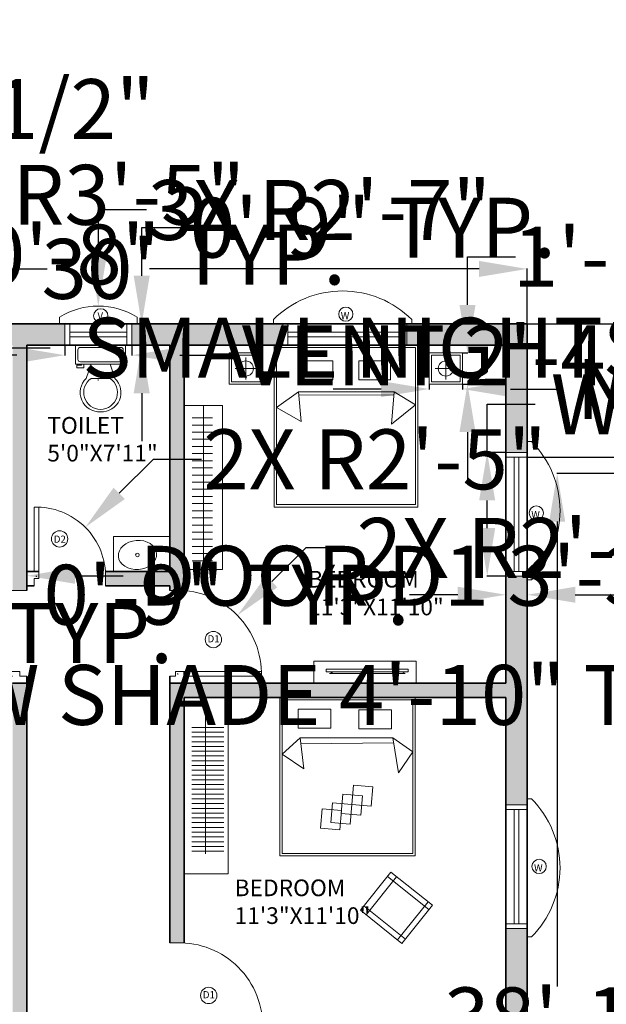
# Model space of a CAD drawing. Units: inches. Extents: x 28 to 3832, y 2 to 1709.
# Tile 4 of 7: x 2710 to 2956, y 1296 to 1709. Entities that reach past the tile are written whole.
import ezdxf

# ---------------------------------------------------------------- set-up
doc = ezdxf.new("R2010")
doc.units = ezdxf.units.IN
doc.header["$MEASUREMENT"] = 0
for name, color, linetype, lineweight in [('A-ANNO-DIMS', 2, 'Continuous', 18), ('A-ANNO-SYMB', 7, 'Continuous', 13), ('A-AREA-IDEN', 7, 'Continuous', 18), ('A-DOOR', 3, 'Continuous', 18), ('A-FLOR-CASE', 8, 'Continuous', 18), ('A-FLOR-CASE-PATT', 8, 'Continuous', 13), ('A-FLOR-FIXT', 9, 'Continuous', 18), ('A-FURN', 8, 'Continuous', 18), ('A-GLAZ', 4, 'Continuous', 18), ('A-ROOF-SHAD', 7, 'Continuous', 13), ('A-WALL', 7, 'Continuous', 35)]:
    doc.layers.add(name, color=color, linetype=linetype, lineweight=lineweight)
doc.layers.add('A-WALL-PATT', color=30, linetype='Continuous', lineweight=9, true_color=0xf26722)
doc.styles.get("Standard").update_dxf_attribs({"font": 'arial.ttf'})
doc.dimstyles.get("Standard").update_dxf_attribs({"dimtxt": 25.18, "dimasz": 20.18, "dimexe": 0.18, "dimexo": 0.0625, "dimgap": 0.09, "dimtad": 0, "dimtih": 1, "dimtoh": 1, "dimdec": 0, "dimzin": 0, "dimdsep": 46, "dimlunit": 3, "dimtxsty": 'Standard', "dimcen": 0.09, "dimadec": 0, "dimazin": 0, "dimtfac": 1, "dimtdec": 0, "dimtofl": 0, "dimtmove": 0, "dimatfit": 3, "dimfxl": 1, "dimtolj": 1, "dimtzin": 0, "dimarcsym": 0})

# ---------------------------------------------------------------- blocks, each defined once
blk = doc.blocks.new('*D1')
at = {"layer": 'A-ANNO-DIMS', "color": 0, "lineweight": -2, "transparency": 16777216}
for p, q in [((2562.64, 1581.59), (2562.64, 1604.74)), ((2582.82, 1604.56), (2721.19, 1604.56)), ((2902.46, 1604.56), (2764.09, 1604.56)), ((2922.64, 1581.59), (2922.64, 1604.74))]:
    blk.add_line(p, q, dxfattribs=at)
at = {"layer": 'A-ANNO-DIMS', "color": 0, "transparency": 16777216}
for points in [[(2582.82, 1607.92), (2582.82, 1601.2), (2562.64, 1604.56)], [(2902.46, 1607.92), (2902.46, 1601.2), (2922.64, 1604.56)]]:
    blk.add_solid(points, dxfattribs=at)
at = {"layer": 'Defpoints', "color": 0, "transparency": 16777216}
for p in [(2922.64, 1604.56), (2562.64, 1581.52), (2922.64, 1581.52)]:
    blk.add_point(p, dxfattribs=at)
at = {"layer": 'A-ANNO-DIMS', "color": 0, "transparency": 16777216, "insert": (2742.64, 1604.56), "char_height": 25.18, "attachment_point": 5}
blk.add_mtext("\\A1;30'", dxfattribs=at)
blk = doc.blocks.new('*U4')
for p, q in [((9.5, -6), (9.5, -2)), ((-8, -8.5), (-8, -8)), ((-7, -8), (-7, -9.5)), ((-4, -8), (-6, -14)), ((4, -8), (6, -14)), ((-10, -8.5), (-8, -8.5)), ((-10, -9.5), (-10, -8.5)), ((-7, -9.5), (-10, -9.5)), ((4, -14), (-4, -14))]:
    blk.add_line(p, q)
blk.add_lwpolyline([(10.5, -8), (10.5, 0), (-10.5, 0), (-10.5, -8)], close=True)
for points in [[(-9.5, -2), (-9.5, -6)], [(8.5, -1), (-8.5, -1)], [(-8.5, -7), (8.5, -7)]]:
    blk.add_lwpolyline(points)
for centre, radius, start, end in [((-8.625, -1.875), 0.8839, 81.8699, 188.1301), ((8.625, -1.875), 0.8839, 351.8699, 98.1301), ((-8.625, -6.125), 0.8839, 171.869898, 278.1301), ((8.625, -6.125), 0.8839, 261.8699, 8.1301), ((-0.4772, -19.9188), 8.0953, 133.01722, 273.38), ((0.0374, -19.8731), 7.127, 124.50543, 269.7), ((-0.0373, -19.8731), 7.127, 270.3, 55.4946), ((0.4773, -19.9188), 8.0953, 266.62, 46.9828)]:
    blk.add_arc(centre, radius, start, end)
blk = doc.blocks.new('DOOR-D1-36')
for p, q in [((33.01, 36), (39.01, 36)), ((36.01, 2), (0.01, 2)), ((33.01, 0), (0.01, 0)), ((36.01, 2), (36.01, 0)), ((36.01, 0), (39.01, 0))]:
    blk.add_line(p, q)
blk.add_arc((35.01, 1), 35.01, 88.3634, 181.6366)
blk = doc.blocks.new('DOOR-D2-30')
for p, q in [((0, 6), (0, 33)), ((2, 3), (2, 33)), ((30, 6), (30, 0)), ((2, 3), (0, 3)), ((0, 3), (0, 0))]:
    blk.add_line(p, q)
blk.add_arc((1, 4), 29.02, 358.0251, 91.9749)
blk = doc.blocks.new('WINDOW-48')
for p, q in [((0, 0), (0, 9)), ((2, 0), (2, 9)), ((50, 0), (50, 9)), ((52, 0), (52, 9)), ((2, 5.5), (50, 5.5)), ((2, 3.5), (50, 3.5))]:
    blk.add_line(p, q)
blk = doc.blocks.new('VENT-24')
for p, q in [((0, 0), (0, 9)), ((2, 0), (2, 9)), ((26, 0), (26, 9)), ((28, 0), (28, 9)), ((2, 5.5), (26, 5.5)), ((2, 3.5), (26, 3.5))]:
    blk.add_line(p, q)
blk = doc.blocks.new('WINDOW-SHADE')
for p, q in [((0, 1.76), (0, 0)), ((58.03, 1.76), (58.03, 0))]:
    blk.add_line(p, q)
blk.add_arc((29.02, -27.22), 41.01, 44.9571, 135.0429)
blk = doc.blocks.new('VENT-SHADE')
for p, q in [((0, 2.83), (0, 0)), ((32.5, 2.83), (32.5, 0))]:
    blk.add_line(p, q)
blk.add_arc((16.25, -23.61), 31.04, 58.4311, 121.5689)
blk = doc.blocks.new('BEDSIDE-TABLE')
for p, q in [((6.98, 11.18), (6.98, 1.93)), ((2.5, 6.54), (11.72, 6.54))]:
    blk.add_line(p, q)
for points in [[(0, 13.08), (13.97, 13.08), (13.97, 0), (0, 0)], [(1, 12.08), (12.97, 12.08), (12.97, 1), (1, 1)]]:
    blk.add_lwpolyline(points, close=True)
blk.add_circle((6.98, 6.54), 3.18)
blk = doc.blocks.new('OPENING-TAG-W')
blk.add_circle((3, 3), 3)
at = {"insert": (0.88, 3.88), "char_height": 3, "attachment_point": 1}
blk.add_mtext_dynamic_manual_height_columns('W', width=16.2124, gutter_width=1, heights=[0], dxfattribs=at)
blk = doc.blocks.new('OPENING-TAG-V')
blk.add_circle((3, 3), 3)
at = {"insert": (1.61, 4.52), "char_height": 3, "attachment_point": 1}
blk.add_mtext_dynamic_manual_height_columns('V', width=16.2124, gutter_width=1, heights=[0], dxfattribs=at)
blk = doc.blocks.new('OPENING-TAG-D1')
blk.add_circle((3.43, 3.43), 3.43)
at = {"insert": (0.97, 5.25), "char_height": 3, "attachment_point": 1}
blk.add_mtext_dynamic_manual_height_columns('D1', width=16.2124, gutter_width=1, heights=[0], dxfattribs=at)
blk = doc.blocks.new('OPENING-TAG-D2')
blk.add_circle((3.43, 3.43), 3.43)
at = {"insert": (0.96, 4.81), "char_height": 3, "attachment_point": 1}
blk.add_mtext_dynamic_manual_height_columns('D2', width=16.2124, gutter_width=1, heights=[0], dxfattribs=at)
blk = doc.blocks.new('*D23')
at = {"layer": 'A-ANNO-DIMS', "color": 0, "lineweight": -2, "transparency": 16777216}
for p, q in [((2540.14, 1405.47), (2540.14, 1425.65)), ((2540.14, 1425.65), (2560.32, 1425.65)), ((2548.79, 1405.47), (2539.96, 1405.47)), ((2540.14, 1367.62), (2540.14, 1385.29)), ((2548.79, 1347.44), (2539.96, 1347.44))]:
    blk.add_line(p, q, dxfattribs=at)
at = {"layer": 'A-ANNO-DIMS', "color": 0, "transparency": 16777216}
for points in [[(2536.78, 1385.29), (2543.51, 1385.29), (2540.14, 1405.47)], [(2536.78, 1367.62), (2543.51, 1367.62), (2540.14, 1347.44)]]:
    blk.add_solid(points, dxfattribs=at)
at = {"layer": 'Defpoints', "color": 0, "transparency": 16777216}
for p in [(2540.14, 1405.47), (2548.85, 1405.47), (2548.85, 1347.44)]:
    blk.add_point(p, dxfattribs=at)
at = {"layer": 'A-ANNO-DIMS', "color": 0, "transparency": 16777216, "insert": (2795, 1425.65), "char_height": 25.18, "attachment_point": 5}
blk.add_mtext('\\A1;WINDOW SHADE 4\'-10" TYP.', dxfattribs=at)
blk = doc.blocks.new('*D25')
at = {"layer": 'A-ANNO-DIMS', "color": 0, "lineweight": -2, "transparency": 16777216}
for p, q in [((2905.84, 1527.52), (2905.84, 1547.7)), ((2905.84, 1547.7), (2926.02, 1547.7)), ((2913.58, 1527.52), (2905.66, 1527.52)), ((2905.84, 1495.7), (2905.84, 1507.34)), ((2913.58, 1475.52), (2905.66, 1475.52))]:
    blk.add_line(p, q, dxfattribs=at)
at = {"layer": 'A-ANNO-DIMS', "color": 0, "transparency": 16777216}
for points in [[(2902.48, 1507.34), (2909.2, 1507.34), (2905.84, 1527.52)], [(2902.48, 1495.7), (2909.2, 1495.7), (2905.84, 1475.52)]]:
    blk.add_solid(points, dxfattribs=at)
at = {"layer": 'Defpoints', "color": 0, "transparency": 16777216}
for p in [(2905.84, 1527.52), (2913.64, 1527.52), (2913.64, 1475.52)]:
    blk.add_point(p, dxfattribs=at)
at = {"layer": 'A-ANNO-DIMS', "color": 0, "transparency": 16777216, "insert": (3085.42, 1547.7), "char_height": 25.18, "attachment_point": 5}
blk.add_mtext('\\A1;WINDOW 4\'-4" TYP.', dxfattribs=at)
blk = doc.blocks.new('*D26')
at = {"layer": 'A-ANNO-DIMS', "color": 0, "lineweight": -2, "transparency": 16777216}
for p, q in [((2913.64, 1475.46), (2913.64, 1467.54)), ((2922.64, 1475.46), (2922.64, 1467.54)), ((2893.46, 1467.72), (2873.28, 1467.72)), ((2942.82, 1467.72), (2963, 1467.72))]:
    blk.add_line(p, q, dxfattribs=at)
at = {"layer": 'A-ANNO-DIMS', "color": 0, "transparency": 16777216}
for points in [[(2893.46, 1471.09), (2893.46, 1464.36), (2913.64, 1467.72)], [(2942.82, 1471.09), (2942.82, 1464.36), (2922.64, 1467.72)]]:
    blk.add_solid(points, dxfattribs=at)
at = {"layer": 'Defpoints', "color": 0, "transparency": 16777216}
for p in [(2913.64, 1475.52), (2922.64, 1475.52), (2913.64, 1467.72)]:
    blk.add_point(p, dxfattribs=at)
at = {"layer": 'A-ANNO-DIMS', "color": 0, "transparency": 16777216, "insert": (2796.45, 1467.72), "char_height": 25.18, "attachment_point": 5}
blk.add_mtext('\\A1;0\'-9" TYP.', dxfattribs=at)
blk = doc.blocks.new('*D31')
at = {"layer": 'A-ANNO-DIMS', "color": 0, "lineweight": -2, "transparency": 16777216}
for p, q in [((2653.18, 1475.69), (2633, 1475.69)), ((2673.36, 1469.86), (2673.36, 1475.87)), ((2712.64, 1469.86), (2712.64, 1475.87)), ((2732.82, 1475.69), (2753, 1475.69))]:
    blk.add_line(p, q, dxfattribs=at)
at = {"layer": 'A-ANNO-DIMS', "color": 0, "transparency": 16777216}
for points in [[(2653.18, 1479.05), (2653.18, 1472.33), (2673.36, 1475.69)], [(2732.82, 1479.05), (2732.82, 1472.33), (2712.64, 1475.69)]]:
    blk.add_solid(points, dxfattribs=at)
at = {"layer": 'Defpoints', "color": 0, "transparency": 16777216}
for p in [(2712.64, 1475.69), (2673.36, 1469.8), (2712.64, 1469.8)]:
    blk.add_point(p, dxfattribs=at)
at = {"layer": 'A-ANNO-DIMS', "color": 0, "transparency": 16777216, "insert": (2943.56, 1475.69), "char_height": 25.18, "attachment_point": 5}
blk.add_mtext('\\A1;DOOR D1 3\'-3 1/2" TYP.', dxfattribs=at)
blk = doc.blocks.new('*D32')
at = {"layer": 'A-ANNO-DIMS', "color": 0, "lineweight": -2, "transparency": 16777216}
for p, q in [((2667.47, 1489.98), (2667.47, 1510.16)), ((2673.3, 1469.8), (2667.29, 1469.8)), ((2673.3, 1433.52), (2667.29, 1433.52)), ((2667.47, 1413.34), (2667.47, 1393.16))]:
    blk.add_line(p, q, dxfattribs=at)
at = {"layer": 'A-ANNO-DIMS', "color": 0, "transparency": 16777216}
for points in [[(2664.11, 1489.98), (2670.84, 1489.98), (2667.47, 1469.8)], [(2664.11, 1413.34), (2670.84, 1413.34), (2667.47, 1433.52)]]:
    blk.add_solid(points, dxfattribs=at)
at = {"layer": 'Defpoints', "color": 0, "transparency": 16777216}
for p in [(2667.47, 1469.8), (2673.36, 1469.8), (2673.36, 1433.52)]:
    blk.add_point(p, dxfattribs=at)
at = {"layer": 'A-ANNO-DIMS', "color": 0, "transparency": 16777216, "insert": (2667.47, 1451.66), "char_height": 25.18, "attachment_point": 5}
blk.add_mtext('\\A1;3\'-0 1/2" TYP.', dxfattribs=at)
blk = doc.blocks.new('*D35')
at = {"layer": 'A-ANNO-DIMS', "color": 0, "lineweight": -2, "transparency": 16777216}
for p, q in [((2728.64, 1572.46), (2728.64, 1568.14)), ((2756.64, 1572.46), (2756.64, 1568.14)), ((2708.46, 1568.32), (2688.28, 1568.32)), ((2776.82, 1568.32), (2797, 1568.32))]:
    blk.add_line(p, q, dxfattribs=at)
at = {"layer": 'A-ANNO-DIMS', "color": 0, "transparency": 16777216}
for points in [[(2708.46, 1571.69), (2708.46, 1564.96), (2728.64, 1568.32)], [(2776.82, 1571.69), (2776.82, 1564.96), (2756.64, 1568.32)]]:
    blk.add_solid(points, dxfattribs=at)
at = {"layer": 'Defpoints', "color": 0, "transparency": 16777216}
for p in [(2728.64, 1572.52), (2756.64, 1572.52), (2756.64, 1568.32)]:
    blk.add_point(p, dxfattribs=at)
at = {"layer": 'A-ANNO-DIMS', "color": 0, "transparency": 16777216, "insert": (2926.28, 1568.32), "char_height": 25.18, "attachment_point": 5}
blk.add_mtext('\\A1;VENT 2\'-4" TYP.', dxfattribs=at)
blk = doc.blocks.new('*D36')
at = {"layer": 'A-ANNO-DIMS', "color": 0, "lineweight": -2, "transparency": 16777216}
for p, q in [((2760.84, 1601.7), (2760.84, 1621.88)), ((2760.84, 1621.88), (2781.02, 1621.88)), ((2756.7, 1581.52), (2761.02, 1581.52)), ((2756.7, 1572.52), (2761.02, 1572.52)), ((2760.84, 1552.34), (2760.84, 1532.16))]:
    blk.add_line(p, q, dxfattribs=at)
at = {"layer": 'A-ANNO-DIMS', "color": 0, "transparency": 16777216}
for points in [[(2757.48, 1601.7), (2764.2, 1601.7), (2760.84, 1581.52)], [(2757.48, 1552.34), (2764.2, 1552.34), (2760.84, 1572.52)]]:
    blk.add_solid(points, dxfattribs=at)
at = {"layer": 'Defpoints', "color": 0, "transparency": 16777216}
for p in [(2756.64, 1581.52), (2760.84, 1581.52), (2756.64, 1572.52)]:
    blk.add_point(p, dxfattribs=at)
at = {"layer": 'A-ANNO-DIMS', "color": 0, "transparency": 16777216, "insert": (2857.85, 1621.88), "char_height": 25.18, "attachment_point": 5}
blk.add_mtext('\\A1;0\'-9" TYP.', dxfattribs=at)
blk = doc.blocks.new('*D39')
at = {"layer": 'A-ANNO-DIMS', "color": 0, "lineweight": -2, "transparency": 16777216}
for p, q in [((2653.75, 1571.46), (2633.57, 1571.46)), ((2673.93, 1570.3), (2673.93, 1571.64)), ((2682.13, 1570.3), (2682.13, 1571.64)), ((2702.31, 1571.46), (2722.49, 1571.46))]:
    blk.add_line(p, q, dxfattribs=at)
at = {"layer": 'A-ANNO-DIMS', "color": 0, "transparency": 16777216}
for points in [[(2653.75, 1574.83), (2653.75, 1568.1), (2673.93, 1571.46)], [(2702.31, 1574.83), (2702.31, 1568.1), (2682.13, 1571.46)]]:
    blk.add_solid(points, dxfattribs=at)
at = {"layer": 'Defpoints', "color": 0, "transparency": 16777216}
for p in [(2682.13, 1571.46), (2673.93, 1570.23), (2682.13, 1570.23)]:
    blk.add_point(p, dxfattribs=at)
at = {"layer": 'A-ANNO-DIMS', "color": 0, "transparency": 16777216, "insert": (2981.04, 1571.46), "char_height": 25.18, "attachment_point": 5}
blk.add_mtext('\\A1;SMALL NIGHTSTAND 0\'-8" TYP.', dxfattribs=at)
blk = doc.blocks.new('*D40')
at = {"layer": 'A-ANNO-DIMS', "color": 0, "lineweight": -2, "transparency": 16777216}
for p, q in [((2672.7, 1590.41), (2672.7, 1610.59)), ((2672.7, 1610.59), (2692.88, 1610.59)), ((2673.87, 1570.23), (2672.52, 1570.23)), ((2673.87, 1562.04), (2672.52, 1562.04)), ((2672.7, 1541.86), (2672.7, 1521.68))]:
    blk.add_line(p, q, dxfattribs=at)
at = {"layer": 'A-ANNO-DIMS', "color": 0, "transparency": 16777216}
for points in [[(2669.34, 1590.41), (2676.07, 1590.41), (2672.7, 1570.23)], [(2669.34, 1541.86), (2676.07, 1541.86), (2672.7, 1562.04)]]:
    blk.add_solid(points, dxfattribs=at)
at = {"layer": 'Defpoints', "color": 0, "transparency": 16777216}
for p in [(2672.7, 1570.23), (2673.93, 1570.23), (2673.93, 1562.04)]:
    blk.add_point(p, dxfattribs=at)
at = {"layer": 'A-ANNO-DIMS', "color": 0, "transparency": 16777216, "insert": (2769.71, 1610.59), "char_height": 25.18, "attachment_point": 5}
blk.add_mtext('\\A1;0\'-8" TYP.', dxfattribs=at)
blk = doc.blocks.new('*D41')
at = {"layer": 'A-ANNO-DIMS', "color": 0, "lineweight": -2, "transparency": 16777216}
for p, q in [((2881.52, 1556.14), (2881.52, 1553.93)), ((2895.49, 1556.14), (2895.49, 1553.93)), ((2861.34, 1554.11), (2841.16, 1554.11)), ((2915.67, 1554.11), (2935.85, 1554.11))]:
    blk.add_line(p, q, dxfattribs=at)
at = {"layer": 'A-ANNO-DIMS', "color": 0, "transparency": 16777216}
for points in [[(2861.34, 1557.47), (2861.34, 1550.74), (2881.52, 1554.11)], [(2915.67, 1557.47), (2915.67, 1550.74), (2895.49, 1554.11)]]:
    blk.add_solid(points, dxfattribs=at)
at = {"layer": 'Defpoints', "color": 0, "transparency": 16777216}
for p in [(2881.52, 1556.2), (2895.49, 1556.2), (2895.49, 1554.11)]:
    blk.add_point(p, dxfattribs=at)
at = {"layer": 'A-ANNO-DIMS', "color": 0, "transparency": 16777216, "insert": (3131.28, 1554.11), "char_height": 25.18, "attachment_point": 5}
blk.add_mtext('\\A1;NIGHTSTAND 1\'-2" TYP.', dxfattribs=at)
blk = doc.blocks.new('*D42')
at = {"layer": 'A-ANNO-DIMS', "color": 0, "lineweight": -2, "transparency": 16777216}
for p, q in [((2897.58, 1589.46), (2897.58, 1609.64)), ((2897.58, 1609.64), (2917.76, 1609.64)), ((2895.55, 1569.28), (2897.76, 1569.28)), ((2895.55, 1556.2), (2897.76, 1556.2)), ((2897.58, 1536.02), (2897.58, 1515.84))]:
    blk.add_line(p, q, dxfattribs=at)
at = {"layer": 'A-ANNO-DIMS', "color": 0, "transparency": 16777216}
for points in [[(2894.22, 1589.46), (2900.95, 1589.46), (2897.58, 1569.28)], [(2894.22, 1536.02), (2900.95, 1536.02), (2897.58, 1556.2)]]:
    blk.add_solid(points, dxfattribs=at)
at = {"layer": 'Defpoints', "color": 0, "transparency": 16777216}
for p in [(2895.49, 1569.28), (2897.58, 1569.28), (2895.49, 1556.2)]:
    blk.add_point(p, dxfattribs=at)
at = {"layer": 'A-ANNO-DIMS', "color": 0, "transparency": 16777216, "insert": (2993.41, 1609.64), "char_height": 25.18, "attachment_point": 5}
blk.add_mtext('\\A1;1\'-1" TYP.', dxfattribs=at)
blk = doc.blocks.new('*D50')
at = {"layer": 'A-ANNO-DIMS', "color": 0, "lineweight": -2, "transparency": 16777216}
for p, q in [((2562.64, 1581.59), (2562.64, 1671.85)), ((2582.82, 1671.67), (2594.96, 1671.67)), ((2615.14, 1581.59), (2615.14, 1671.85)), ((2615.14, 1671.67), (2635.32, 1671.67))]:
    blk.add_line(p, q, dxfattribs=at)
at = {"layer": 'A-ANNO-DIMS', "color": 0, "transparency": 16777216}
for points in [[(2582.82, 1675.04), (2582.82, 1668.31), (2562.64, 1671.67)], [(2594.96, 1675.04), (2594.96, 1668.31), (2615.14, 1671.67)]]:
    blk.add_solid(points, dxfattribs=at)
at = {"layer": 'Defpoints', "color": 0, "transparency": 16777216}
for p in [(2615.14, 1671.67), (2562.64, 1581.52), (2615.14, 1581.52)]:
    blk.add_point(p, dxfattribs=at)
at = {"layer": 'A-ANNO-DIMS', "color": 0, "transparency": 16777216, "insert": (2698.72, 1671.67), "char_height": 25.18, "attachment_point": 5}
blk.add_mtext('\\A1;4\'-4 1/2"', dxfattribs=at)
blk = doc.blocks.new('*D51')
at = {"layer": 'A-ANNO-DIMS', "color": 0, "lineweight": -2, "transparency": 16777216}
for p, q in [((2975.53, 1581.52), (2975.53, 1601.7)), ((2975.53, 1601.7), (2995.71, 1601.7)), ((2922.7, 1581.52), (2975.71, 1581.52)), ((2975.53, 1545.7), (2975.53, 1561.34)), ((2922.7, 1525.52), (2975.71, 1525.52))]:
    blk.add_line(p, q, dxfattribs=at)
at = {"layer": 'A-ANNO-DIMS', "color": 0, "transparency": 16777216}
for points in [[(2972.16, 1561.34), (2978.89, 1561.34), (2975.53, 1581.52)], [(2972.16, 1545.7), (2978.89, 1545.7), (2975.53, 1525.52)]]:
    blk.add_solid(points, dxfattribs=at)
at = {"layer": 'Defpoints', "color": 0, "transparency": 16777216}
for p in [(2922.64, 1581.52), (2975.53, 1581.52), (2922.64, 1525.52)]:
    blk.add_point(p, dxfattribs=at)
at = {"layer": 'A-ANNO-DIMS', "color": 0, "transparency": 16777216, "insert": (3029.77, 1601.7), "char_height": 25.18, "attachment_point": 5}
blk.add_mtext('\\A1;4\'-8"', dxfattribs=at)
blk = doc.blocks.new('*D54')
at = {"layer": 'A-ANNO-DIMS', "color": 0, "lineweight": -2, "transparency": 16777216}
for p, q in [((3022.59, 1518.63), (2935.04, 1518.63)), ((2935.22, 1498.45), (2935.22, 1303.17)), ((2935.22, 1081.98), (2935.22, 1277.26)), ((2960.61, 1061.8), (2935.04, 1061.8))]:
    blk.add_line(p, q, dxfattribs=at)
at = {"layer": 'A-ANNO-DIMS', "color": 0, "transparency": 16777216}
for points in [[(2931.86, 1498.45), (2938.58, 1498.45), (2935.22, 1518.63)], [(2931.86, 1081.98), (2938.58, 1081.98), (2935.22, 1061.8)]]:
    blk.add_solid(points, dxfattribs=at)
at = {"layer": 'Defpoints', "color": 0, "transparency": 16777216}
for p in [(2935.22, 1518.63), (3022.65, 1518.63), (2960.67, 1061.8)]:
    blk.add_point(p, dxfattribs=at)
at = {"layer": 'A-ANNO-DIMS', "color": 0, "transparency": 16777216, "insert": (2935.22, 1290.21), "char_height": 25.18, "attachment_point": 5}
blk.add_mtext('\\A1;38\'-1"', dxfattribs=at)
blk = doc.blocks.new('*D67')
at = {"layer": 'A-ANNO-DIMS', "color": 0, "lineweight": -2, "transparency": 16777216}
for p, q in [((2659.56, 1635.67), (2639.38, 1635.67)), ((2639.38, 1635.67), (2639.38, 1615.49)), ((2639.29, 1554.31), (2639.47, 1554.31)), ((2639.38, 1554.22), (2639.38, 1554.4))]:
    blk.add_line(p, q, dxfattribs=at)
at = {"layer": 'A-ANNO-DIMS', "color": 0, "transparency": 16777216}
blk.add_solid([(2636.01, 1615.49), (2642.74, 1615.49), (2639.38, 1595.31)], dxfattribs=at)
at = {"layer": 'Defpoints', "color": 0, "transparency": 16777216}
for p in [(2639.38, 1595.31), (2639.38, 1554.31)]:
    blk.add_point(p, dxfattribs=at)
at = {"layer": 'A-ANNO-DIMS', "color": 0, "transparency": 16777216, "insert": (2732.23, 1635.67), "char_height": 25.18, "attachment_point": 5}
blk.add_mtext('\\A1;8X R3\'-5"', dxfattribs=at)
blk = doc.blocks.new('*D68')
at = {"layer": 'A-ANNO-DIMS', "color": 0, "lineweight": -2, "transparency": 16777216}
for p, q in [((2762.81, 1629.31), (2742.63, 1629.31)), ((2742.63, 1629.31), (2742.63, 1609.13)), ((2742.54, 1557.91), (2742.72, 1557.91)), ((2742.63, 1557.82), (2742.63, 1558))]:
    blk.add_line(p, q, dxfattribs=at)
at = {"layer": 'A-ANNO-DIMS', "color": 0, "transparency": 16777216}
blk.add_solid([(2739.27, 1609.13), (2746, 1609.13), (2742.63, 1588.95)], dxfattribs=at)
at = {"layer": 'Defpoints', "color": 0, "transparency": 16777216}
for p in [(2742.63, 1588.95), (2742.63, 1557.91)]:
    blk.add_point(p, dxfattribs=at)
at = {"layer": 'A-ANNO-DIMS', "color": 0, "transparency": 16777216, "insert": (2835.46, 1629.31), "char_height": 25.18, "attachment_point": 5}
blk.add_mtext('\\A1;3X R2\'-7"', dxfattribs=at)
blk = doc.blocks.new('*D69')
at = {"layer": 'A-ANNO-DIMS', "color": 0, "lineweight": -2, "transparency": 16777216}
for p, q in [((2829.79, 1487.38), (2815.4, 1473.22)), ((2849.97, 1487.38), (2829.79, 1487.38)), ((2775.98, 1434.52), (2776.16, 1434.52)), ((2776.07, 1434.43), (2776.07, 1434.61))]:
    blk.add_line(p, q, dxfattribs=at)
at = {"layer": 'A-ANNO-DIMS', "color": 0, "transparency": 16777216}
blk.add_solid([(2813.05, 1475.62), (2817.76, 1470.83), (2801.02, 1459.07)], dxfattribs=at)
at = {"layer": 'Defpoints', "color": 0, "transparency": 16777216}
for p in [(2801.02, 1459.07), (2776.07, 1434.52)]:
    blk.add_point(p, dxfattribs=at)
at = {"layer": 'A-ANNO-DIMS', "color": 0, "transparency": 16777216, "insert": (2932.62, 1487.38), "char_height": 25.18, "attachment_point": 5}
blk.add_mtext('\\A1;2X R2\'-11"', dxfattribs=at)
blk = doc.blocks.new('*D70')
at = {"layer": 'A-ANNO-DIMS', "color": 0, "lineweight": -2, "transparency": 16777216}
for p, q in [((2765.7, 1524.58), (2751.43, 1510.31)), ((2785.88, 1524.58), (2765.7, 1524.58)), ((2716.55, 1475.52), (2716.73, 1475.52)), ((2716.64, 1475.43), (2716.64, 1475.61))]:
    blk.add_line(p, q, dxfattribs=at)
at = {"layer": 'A-ANNO-DIMS', "color": 0, "transparency": 16777216}
blk.add_solid([(2749.05, 1512.69), (2753.8, 1507.93), (2737.16, 1496.04)], dxfattribs=at)
at = {"layer": 'Defpoints', "color": 0, "transparency": 16777216}
for p in [(2737.16, 1496.04), (2716.64, 1475.52)]:
    blk.add_point(p, dxfattribs=at)
at = {"layer": 'A-ANNO-DIMS', "color": 0, "transparency": 16777216, "insert": (2858.75, 1524.58), "char_height": 25.18, "attachment_point": 5}
blk.add_mtext('\\A1;2X R2\'-5"', dxfattribs=at)

msp = doc.modelspace()

# ---------------------------------------------------------------- hatches: boundary and pattern name
at = {"layer": 'A-FLOR-CASE-PATT'}
h = msp.add_hatch(dxfattribs=at)
h.set_pattern_fill('ANSI31', color=256, scale=24, angle=-45, style=0)
h.paths.add_polyline_path([(2782.05, 1479.03), (2790.49, 1479.03), (2790.49, 1544.97), (2782.05, 1544.97)])
h = msp.add_hatch(dxfattribs=at)
h.set_pattern_fill('ANSI31', color=256, scale=16, angle=-45, style=0)
h.paths.add_polyline_path([(2781.82, 1359.04), (2795.26, 1359.04), (2795.26, 1413), (2781.82, 1413)])
at = {"layer": 'A-WALL-PATT'}
h = msp.add_hatch(color=256, dxfattribs=at)
h.dxf.hatch_style = 1
h.paths.add_polyline_path([(2571.64, 1572.52), (2613.14, 1572.52), (2613.14, 1581.52), (2562.64, 1581.52), (2562.64, 1527.52), (2571.64, 1527.52)])
h.paths.add_polyline_path([(2728.64, 1581.52), (2665.14, 1581.52), (2665.14, 1572.52), (2670.22, 1572.52), (2706.64, 1572.52), (2706.64, 1469.52), (2707.64, 1469.52, -0.014283), (2709.64, 1469.52), (2712.64, 1469.52), (2712.64, 1471.52), (2712.64, 1477.52), (2712.64, 1572.52), (2728.64, 1572.52)])
h.paths.add_polyline_path([(2820.14, 1581.52), (2756.64, 1581.52), (2756.64, 1572.52), (2772.64, 1572.52), (2772.64, 1477.52), (2745.64, 1477.52), (2745.64, 1476.52, -0.017236), (2745.64, 1474.52), (2745.64, 1471.52), (2772.64, 1471.52), (2772.64, 1469.52), (2775.64, 1469.52, -0.006113), (2776.49, 1469.52), (2778.64, 1469.52), (2778.64, 1572.52), (2820.14, 1572.52)])
h.paths.add_polyline_path([(2922.64, 1581.52), (2872.14, 1581.52), (2872.14, 1572.52), (2913.64, 1572.52), (2913.64, 1527.52), (2922.64, 1527.52)])
h.paths.add_polyline_path([(2922.64, 1475.52), (2913.64, 1475.52), (2913.64, 1430.52), (2778.64, 1430.52), (2772.64, 1430.52), (2772.64, 1321.52), (2775.64, 1321.52, -0.014283), (2777.64, 1321.52), (2778.64, 1321.52), (2778.64, 1424.52), (2913.64, 1424.52), (2913.64, 1379.52), (2922.64, 1379.52)])
h.paths.add_polyline_path([(2571.64, 1475.52), (2562.64, 1475.52), (2562.64, 1402.52), (2571.64, 1402.52), (2571.64, 1424.52), (2706.64, 1424.52), (2706.64, 1328.52), (2706.64, 1322.52), (2706.64, 1290.16), (2712.64, 1290.16), (2712.64, 1430.52), (2706.64, 1430.52), (2571.64, 1430.52)])
h.paths.add_polyline_path([(2571.64, 1322.52), (2667.64, 1322.52), (2667.64, 1325.52, -0.014283), (2667.64, 1327.52), (2667.64, 1328.52), (2571.64, 1328.52), (2571.64, 1350.52), (2562.64, 1350.52), (2562.64, 1283.02), (2571.64, 1283.02)])
h.paths.add_polyline_path([(2712.64, 1241.01), (2706.64, 1241.01), (2706.64, 1191.52), (2571.64, 1191.52), (2571.64, 1231.02), (2562.64, 1231.02), (2562.64, 1172.52), (2571.64, 1172.52), (2571.64, 1185.52), (2706.64, 1185.52), (2712.64, 1185.52)])
h.paths.add_polyline_path([(2571.64, 1125.52), (2712.64, 1125.52), (2719.5, 1125.52), (2719.5, 1128.52), (2721.5, 1128.52), (2721.5, 1131.52), (2571.64, 1131.52), (2571.64, 1144.52), (2562.64, 1144.52), (2562.64, 1041.52), (2740.31, 1041.52), (2740.31, 1050.52), (2571.64, 1050.52)])
h.paths.add_polyline_path([(2712.64, 1152.52), (2709.64, 1152.52, -0.017236), (2707.64, 1152.52), (2706.64, 1152.52), (2706.64, 1131.52), (2712.64, 1131.52)])
h.paths.add_polyline_path([(2922.64, 1178.52), (2913.64, 1178.52), (2913.64, 1132.52), (2922.64, 1132.52)], flags=17)
h.paths.add_polyline_path([(2922.64, 1327.52), (2913.64, 1327.52), (2913.64, 1282.52), (2772.64, 1282.52), (2772.64, 1276.52), (2778.64, 1276.52), (2913.64, 1276.52), (2913.64, 1230.52), (2922.64, 1230.52)])
edge = h.paths.add_edge_path()
edge.add_line((2880.64, 1132.52), (2772.64, 1132.52))
edge.add_line((2772.64, 1132.52), (2772.64, 1126.52))
edge.add_line((2772.64, 1126.52), (2853.64, 1126.52))
edge.add_line((2853.64, 1126.52), (2853.64, 1050.52))
edge.add_line((2853.64, 1050.52), (2835.37, 1050.52))
edge.add_line((2835.37, 1050.52), (2835.37, 1041.52))
edge.add_line((2835.37, 1041.52), (2922.64, 1041.52))
edge.add_line((2922.64, 1041.52), (2922.64, 1074.52))
edge.add_line((2922.64, 1074.52), (2913.64, 1074.52))
edge.add_line((2913.64, 1074.52), (2913.64, 1050.52))
edge.add_line((2913.64, 1050.52), (2859.64, 1050.52))
edge.add_line((2859.64, 1050.52), (2859.64, 1126.52))
edge.add_line((2859.64, 1126.52), (2880.64, 1126.52))
edge.add_line((2880.64, 1126.52), (2880.64, 1127.52))
edge.add_arc((2909.64, 1128.52), 29.02, 178.0251, 181.9749, ccw=False)
edge.add_line((2880.64, 1129.52), (2880.64, 1132.52))

# ---------------------------------------------------------------- linework, layer by layer
at = {"layer": 'A-DOOR'}
for p, q in [((2778.64, 1469.52), (2772.64, 1469.52)), ((2775.05, 1435.52), (2775.05, 1433.52)), ((2775.05, 1433.52), (2772.64, 1433.52))]:
    msp.add_line(p, q, dxfattribs=at)
for points in [[(2775.05, 1435.52), (2811.05, 1435.52)], [(2778.64, 1433.52), (2811.05, 1433.52)]]:
    msp.add_lwpolyline(points, dxfattribs=at)
msp.add_arc((2776.07, 1434.52), 35, 358.3629, 90.7005, dxfattribs=at)
at = {"layer": 'A-FLOR-CASE'}
for p, q in [((2786.71, 1547.15), (2786.71, 1478.26)), ((2797.13, 1424.52), (2797.13, 1350.54)), ((2787.59, 1416.63), (2787.59, 1358.85)), ((2797.13, 1350.54), (2778.64, 1350.54))]:
    msp.add_line(p, q, dxfattribs=at)
msp.add_lwpolyline([(2778.64, 1547.15), (2794.77, 1547.15), (2794.77, 1478.26), (2778.64, 1478.26)], close=True, dxfattribs=at)
at = {"layer": 'A-FLOR-FIXT'}
for p, q in [((2748.99, 1477.52), (2748.99, 1492.21)), ((2748.99, 1492.21), (2772.64, 1492.21))]:
    msp.add_line(p, q, dxfattribs=at)
msp.add_circle((2759.06, 1484.43), 0.754, dxfattribs=at)
msp.add_ellipse((2759.06, 1484.43), major_axis=(8.02, 0.63), ratio=0.76056, start_param=-1.570796, end_param=4.712389, dxfattribs=at)
at = {"layer": 'A-FURN'}
for p, q in [((2826.65, 1552.94), (2817.47, 1546.37)), ((2826.65, 1552.94), (2866.82, 1552.94)), ((2827.76, 1540.43), (2826.65, 1552.94)), ((2826.78, 1551.53), (2866.72, 1551.68)), ((2865.75, 1539.39), (2866.82, 1552.94)), ((2866.82, 1552.94), (2875.75, 1547.47)), ((2875.75, 1547.47), (2865.75, 1539.39)), ((2817.47, 1546.37), (2827.76, 1540.43)), ((2841.49, 1435.31), (2839.72, 1434.62)), ((2871.45, 1434.62), (2870.14, 1435.31)), ((2839.72, 1434.62), (2871.45, 1434.62)), ((2827.29, 1407.67), (2819.76, 1400.7)), ((2827.29, 1407.67), (2866.2, 1407.67)), ((2828.85, 1394.54), (2827.29, 1407.67)), ((2866.2, 1407.67), (2874.58, 1401.71)), ((2868.62, 1392.96), (2866.2, 1407.67)), ((2827.6, 1405.07), (2866.54, 1405.58)), ((2819.76, 1400.7), (2828.85, 1394.54)), ((2874.58, 1401.71), (2868.62, 1392.96)), ((2855.05, 1333.29), (2867.84, 1349.29)), ((2864, 1349.41), (2881.42, 1335.49)), ((2871.51, 1323.08), (2854.08, 1337.01)), ((2881.01, 1338.77), (2868.22, 1322.76))]:
    msp.add_line(p, q, dxfattribs=at)
for points in [[(2816.47, 1572.52), (2876.75, 1572.52), (2876.75, 1504.56), (2816.47, 1504.56)], [(2817.47, 1571.52), (2875.75, 1571.52), (2875.75, 1505.56), (2817.47, 1505.56)], [(2827.77, 1565.92), (2841.04, 1565.92), (2841.04, 1557.93), (2827.77, 1557.93)], [(2851.96, 1565.92), (2865.23, 1565.92), (2865.23, 1557.93), (2851.96, 1557.93)], [(2833.15, 1430.52), (2875.98, 1430.52), (2875.98, 1439.77), (2833.15, 1439.77)], [(2838.33, 1435.31), (2872.74, 1435.31), (2872.74, 1436.53), (2838.33, 1436.53)], [(2818.76, 1424.52), (2875.58, 1424.52), (2875.58, 1358.07), (2818.76, 1358.07)], [(2819.76, 1423.52), (2874.58, 1423.52), (2874.58, 1359.07), (2819.76, 1359.07)], [(2826.57, 1419.7), (2840.24, 1419.7), (2840.24, 1411.67), (2826.57, 1411.67)], [(2852.04, 1419.43), (2865.71, 1419.43), (2865.71, 1411.39), (2852.04, 1411.39)], [(2857.2, 1378.9), (2857.89, 1387.06), (2849.73, 1387.75), (2849.04, 1379.58)], [(2852.78, 1375.16), (2853.47, 1383.32), (2845.3, 1384.01), (2844.62, 1375.85)], [(2844.04, 1368.93), (2844.72, 1377.09), (2836.56, 1377.78), (2835.87, 1369.62)], [(2848.36, 1371.42), (2849.04, 1379.58), (2840.88, 1380.27), (2840.19, 1372.11)], [(2870.08, 1321.29), (2852.65, 1335.21), (2865.43, 1351.21), (2882.86, 1337.29)]]:
    msp.add_lwpolyline(points, close=True, dxfattribs=at)
at = {"layer": 'A-WALL'}
for p, q in [((2562.64, 1581.52), (2922.64, 1581.52)), ((2922.64, 1581.52), (2922.64, 1041.52)), ((2712.64, 1572.52), (2772.64, 1572.52)), ((2712.64, 1477.52), (2712.64, 1572.52)), ((2712.64, 1477.52), (2712.64, 1572.52)), ((2772.64, 1572.52), (2772.64, 1477.52)), ((2772.64, 1477.52), (2772.64, 1572.52)), ((2913.64, 1572.52), (2778.64, 1572.52)), ((2778.64, 1572.52), (2778.64, 1469.43)), ((2778.64, 1572.52), (2913.64, 1572.52)), ((2778.64, 1469.43), (2778.64, 1572.52)), ((2913.64, 1572.52), (2913.64, 1430.52)), ((2712.64, 1477.52), (2717.64, 1477.52)), ((2712.64, 1477.52), (2712.64, 1471.52)), ((2745.59, 1477.52), (2772.64, 1477.52)), ((2712.64, 1471.52), (2715.64, 1471.52)), ((2712.64, 1469.52), (2712.64, 1471.52)), ((2712.64, 1469.52), (2712.64, 1471.52)), ((2745.64, 1471.52), (2772.64, 1471.52)), ((2772.64, 1471.52), (2772.64, 1469.52)), ((2772.64, 1469.52), (2772.64, 1471.52)), ((2778.64, 1430.52), (2778.64, 1435.52)), ((2778.64, 1435.52), (2778.64, 1430.52)), ((2712.64, 1424.52), (2712.64, 1433.52)), ((2712.64, 1290.16), (2712.64, 1433.52)), ((2772.64, 1424.52), (2772.64, 1433.52)), ((2772.64, 1433.52), (2772.64, 1321.52)), ((2706.64, 1430.52), (2712.64, 1430.52)), ((2778.64, 1430.52), (2772.64, 1430.52)), ((2778.64, 1430.52), (2913.64, 1430.52)), ((2778.64, 1424.52), (2913.64, 1424.52)), ((2778.64, 1424.52), (2778.64, 1321.48)), ((2913.64, 1424.52), (2913.64, 1282.52))]:
    msp.add_line(p, q, dxfattribs=at)

# ---------------------------------------------------------------- block references
at = {"layer": 'A-ANNO-SYMB'}
for name, p in [('OPENING-TAG-W', (2843.51, 1582.55)), ('OPENING-TAG-V', (2740.66, 1581.83)), ('OPENING-TAG-W', (2923.47, 1499.01)), ('OPENING-TAG-D2', (2722.97, 1487.75)), ('OPENING-TAG-D1', (2787.51, 1445.48)), ('OPENING-TAG-W', (2924.64, 1350.62)), ('OPENING-TAG-D1', (2785.52, 1295.99))]:
    msp.add_blockref(name, p, dxfattribs=at)
at = {"layer": 'A-DOOR'}
for name, p in [('DOOR-D2-30', (2715.64, 1471.52)), ('DOOR-D1-36', (2673.62, 1433.52))]:
    msp.add_blockref(name, p, dxfattribs=at)
at = {"layer": 'A-DOOR', "extrusion": (0, 0, -1), "zscale": -1}
msp.add_blockref('DOOR-D1-36', (-2811.65, 1285.52), dxfattribs=at)
at = {"layer": 'A-FLOR-FIXT'}
msp.add_blockref('*U4', (2743.59, 1572.57), dxfattribs=at)
at = {"layer": 'A-FURN'}
for p in [(2797.54, 1556.2), (2881.52, 1556.2)]:
    msp.add_blockref('BEDSIDE-TABLE', p, dxfattribs=at)
at = {"layer": 'A-GLAZ'}
for name, p in [('VENT-24', (2728.64, 1572.52)), ('WINDOW-48', (2820.14, 1572.52))]:
    msp.add_blockref(name, p, dxfattribs=at)
for p, rotation in [((2922.64, 1475.52), 89.99999999999886), ((2922.64, 1327.52), 89.99999999999876)]:
    msp.add_blockref('WINDOW-48', p, dxfattribs=dict(at, rotation=rotation))
at = {"layer": 'A-ROOF-SHAD'}
for name, p in [('WINDOW-SHADE', (2816.12, 1581.52)), ('VENT-SHADE', (2726.38, 1581.52))]:
    msp.add_blockref(name, p, dxfattribs=at)
for p, rotation in [((2922.64, 1532.08), 269.9999999999989), ((2922.64, 1382.03), 269.9999999999979)]:
    msp.add_blockref('WINDOW-SHADE', p, dxfattribs=dict(at, rotation=rotation))

# ---------------------------------------------------------------- texts
at = {"layer": 'A-AREA-IDEN', "char_height": 7, "attachment_point": 1}
for s, insert in [('TOILET\\P5\'0"X7\'11"', (2721.23, 1542.35)), ('BEDROOM\\P11\'3"X11\'10"', (2830.68, 1477.75)), ('BEDROOM\\P11\'3"X11\'10"', (2799.85, 1348.13))]:
    msp.add_mtext_dynamic_manual_height_columns(s, width=107.6964, gutter_width=1, heights=[0], dxfattribs=dict(at, insert=insert))

# ---------------------------------------------------------------- dimensions: what is measured, and where the dimension line sits
at = {"layer": 'A-ANNO-DIMS'}
for base, p2, override, picture, middle in [((2615.14, 1671.67), (2615.14, 1581.52), {"dimdec": 1, "dimlfac": 1, "dimrnd": 0, "dimzin": 1, "dimdsep": 46, "dimlunit": 4, "dimfrac": 2}, '*D50', (2698.72, 1671.67)), ((2922.64, 1604.56), (2922.64, 1581.52), {"dimclrd": 0, "dimclre": 0, "dimclrt": 0}, '*D1', (2742.64, 1604.56))]:
    dim = msp.add_linear_dim(base=base, p1=(2562.64, 1581.52), p2=p2, dimstyle='Standard', override=override, dxfattribs=at)
    dim.commit()
    dim.dimension.update_dxf_attribs({"geometry": picture, "text_midpoint": middle})
for center, mpoint, text, picture, middle in [((2639.38, 1554.31), (2639.38, 1595.31), '8X <>', '*D67', (2732.23, 1635.67)), ((2742.63, 1557.91), (2742.63, 1588.95), '3X <>', '*D68', (2835.46, 1629.31)), ((2716.64, 1475.52), (2737.16, 1496.04), '2X <>', '*D70', (2858.75, 1524.58)), ((2776.07, 1434.52), (2801.02, 1459.07), '2X <>', '*D69', (2932.62, 1487.38))]:
    dim = msp.add_radius_dim(center=center, mpoint=mpoint, text=text, dimstyle='Standard', override={"dimdec": 1, "dimlfac": 1, "dimrnd": 0, "dimzin": 1, "dimdsep": 46, "dimlunit": 4, "dimfrac": 2}, dxfattribs=at)
    dim.commit()
    dim.dimension.update_dxf_attribs({"geometry": picture, "text_midpoint": middle})
for base, p1, p2, angle, text, picture, middle in [((2760.84, 1581.52), (2756.64, 1572.52), (2756.64, 1581.52), 90, '<> TYP.', '*D36', (2857.85, 1621.88)), ((2672.7, 1570.23), (2673.93, 1562.04), (2673.93, 1570.23), 90, '<> TYP.', '*D40', (2769.71, 1610.59)), ((2897.58, 1569.28), (2895.49, 1556.2), (2895.49, 1569.28), 90, '<> TYP.', '*D42', (2993.41, 1609.64)), ((2905.84, 1527.52), (2913.64, 1475.52), (2913.64, 1527.52), 90, 'WINDOW <> TYP.', '*D25', (3085.42, 1547.7)), ((2667.47, 1469.8), (2673.36, 1433.52), (2673.36, 1469.8), 90, '<> TYP.', '*D32', (2667.47, 1451.66)), ((2540.14, 1405.47), (2548.85, 1347.44), (2548.85, 1405.47), 90, 'WINDOW SHADE <> TYP.', '*D23', (2795, 1425.65)), ((2913.64, 1467.72), (2922.64, 1475.52), (2913.64, 1475.52), 180, '<> TYP.', '*D26', (2796.45, 1467.72))]:
    dim = msp.add_linear_dim(base=base, p1=p1, p2=p2, angle=angle, text=text, dimstyle='Standard', override={"dimdec": 1, "dimlfac": 1, "dimrnd": 0, "dimzin": 1, "dimdsep": 46, "dimlunit": 4, "dimfrac": 2}, dxfattribs=at)
    dim.commit()
    dim.dimension.update_dxf_attribs({"geometry": picture, "text_midpoint": middle})
for base, p1, p2, text, picture, middle in [((2682.13, 1571.46), (2673.93, 1570.23), (2682.13, 1570.23), 'SMALL NIGHTSTAND <> TYP.', '*D39', (2981.04, 1571.46)), ((2756.64, 1568.32), (2728.64, 1572.52), (2756.64, 1572.52), 'VENT <> TYP.', '*D35', (2926.28, 1568.32)), ((2895.49, 1554.11), (2881.52, 1556.2), (2895.49, 1556.2), 'NIGHTSTAND <> TYP.', '*D41', (3131.28, 1554.11)), ((2712.64, 1475.69), (2673.36, 1469.8), (2712.64, 1469.8), 'DOOR D1 <> TYP.', '*D31', (2943.56, 1475.69))]:
    dim = msp.add_linear_dim(base=base, p1=p1, p2=p2, text=text, dimstyle='Standard', override={"dimdec": 1, "dimlfac": 1, "dimrnd": 0, "dimzin": 1, "dimdsep": 46, "dimlunit": 4, "dimfrac": 2}, dxfattribs=at)
    dim.commit()
    dim.dimension.update_dxf_attribs({"geometry": picture, "text_midpoint": middle})
for base, p1, p2, picture, middle in [((2975.53, 1581.52), (2922.64, 1525.52), (2922.64, 1581.52), '*D51', (3029.77, 1601.7)), ((2935.22, 1518.63), (2960.67, 1061.8), (3022.65, 1518.63), '*D54', (2935.22, 1290.21))]:
    dim = msp.add_linear_dim(base=base, p1=p1, p2=p2, angle=90, dimstyle='Standard', override={"dimdec": 1, "dimlfac": 1, "dimrnd": 0, "dimzin": 1, "dimdsep": 46, "dimlunit": 4, "dimfrac": 2}, dxfattribs=at)
    dim.commit()
    dim.dimension.update_dxf_attribs({"geometry": picture, "text_midpoint": middle})

doc.saveas('drawing.dxf')
